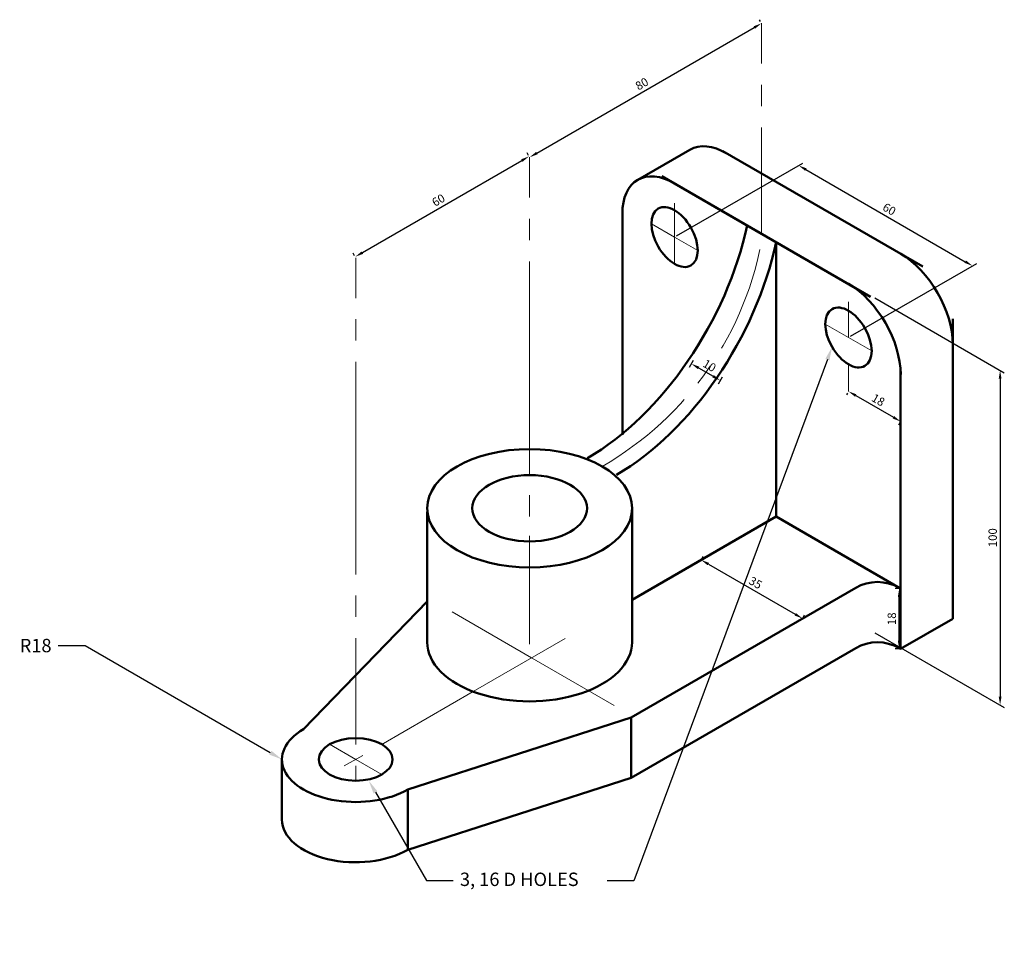
# Model space of a CAD drawing. Units: millimetres. Extents: x 10284 to 10578, y 6421 to 6701.
import ezdxf
from ezdxf import colors
from ezdxf.entities.mleader import LeaderData, LeaderLine
from ezdxf.math import Vec2, Vec3

# ---------------------------------------------------------------- set-up
doc = ezdxf.new("R2010")
doc.units = ezdxf.units.MM
doc.linetypes.add('CENTER', pattern=[50.8, 31.75, -6.35, 6.35, -6.35])
for name, color, linetype, lineweight in [('M-CNTR', 4, 'CENTER', 18), ('M-DIMS', 2, 'Continuous', 25), ('M-OUTL', 7, 'Continuous', 50), ('M-TEXT', 3, 'Continuous', 25)]:
    doc.layers.add(name, color=color, linetype=linetype, lineweight=lineweight)
doc.styles.get("Standard").update_dxf_attribs({"font": 'arial.ttf'})
doc.dimstyles.new('ISO-25', dxfattribs={"dimtxt": 2.5, "dimasz": 2.5, "dimexe": 1.25, "dimexo": 0.625, "dimtad": 1, "dimtxsty": 'Standard', "dimcen": 2.5, "dimadec": 0, "dimazin": 0, "dimtfac": 1, "dimtmove": 0, "dimatfit": 3, "dimfxl": 1, "dimarcsym": 0})

# ---------------------------------------------------------------- blocks, each defined once
blk = doc.blocks.new('*D1')
at = {"layer": 'Defpoints', "color": 0, "transparency": 16777216}
for p in [(10546.86, 6530.7), (10547.29, 6530.7), (10547.29, 6512.7)]:
    blk.add_point(p, dxfattribs=at)
at = {"layer": 'M-DIMS', "color": 0, "lineweight": -2, "transparency": 16777216}
for p, q in [((10546.66, 6530.7), (10545.61, 6530.7)), ((10546.86, 6515.2), (10546.86, 6528.2)), ((10546.66, 6512.7), (10545.61, 6512.7))]:
    blk.add_line(p, q, dxfattribs=at)
at = {"layer": 'M-DIMS', "color": 0, "transparency": 16777216}
for points in [[(10546.44, 6528.2), (10547.28, 6528.2), (10546.86, 6530.7)], [(10546.44, 6515.2), (10547.28, 6515.2), (10546.86, 6512.7)]]:
    blk.add_solid(points, dxfattribs=at)
at = {"layer": 'M-DIMS', "color": 0, "transparency": 16777216, "insert": (10544.96, 6521.7), "char_height": 2.5, "attachment_point": 5, "rotation": 90}
blk.add_mtext('18', dxfattribs=at)
blk = doc.blocks.new('*D2')
at = {"layer": 'Defpoints', "color": 0, "transparency": 16777216}
for p in [(10487.67, 6539.28), (10517.98, 6521.78), (10517.98, 6521.78)]:
    blk.add_point(p, dxfattribs=at)
at = {"layer": 'M-DIMS', "color": 0, "lineweight": -2, "transparency": 16777216}
for p, q in [((10487.98, 6539.82), (10488.29, 6540.36)), ((10489.83, 6538.03), (10515.81, 6523.03)), ((10518.29, 6522.32), (10518.6, 6522.86))]:
    blk.add_line(p, q, dxfattribs=at)
at = {"layer": 'M-DIMS', "color": 0, "transparency": 16777216}
for points in [[(10490.04, 6538.39), (10489.63, 6537.67), (10487.67, 6539.28)], [(10516.02, 6523.39), (10515.61, 6522.67), (10517.98, 6521.78)]]:
    blk.add_solid(points, dxfattribs=at)
at = {"layer": 'M-DIMS', "color": 0, "transparency": 16777216, "insert": (10503.77, 6532.18), "char_height": 2.5, "attachment_point": 5, "rotation": 330}
blk.add_mtext('35', dxfattribs=at)
blk = doc.blocks.new('*D3')
at = {"layer": 'Defpoints', "color": 0, "transparency": 16777216}
for p in [(10531.7, 6589.62), (10547.29, 6580.62), (10547.29, 6580.62)]:
    blk.add_point(p, dxfattribs=at)
at = {"layer": 'M-DIMS', "color": 0, "lineweight": -2, "transparency": 16777216}
for p, q in [((10531.39, 6589.08), (10531.07, 6588.54)), ((10533.86, 6588.37), (10545.12, 6581.87)), ((10546.98, 6580.08), (10546.66, 6579.54))]:
    blk.add_line(p, q, dxfattribs=at)
at = {"layer": 'M-DIMS', "color": 0, "transparency": 16777216}
for points in [[(10534.07, 6588.73), (10533.66, 6588.01), (10531.7, 6589.62)], [(10545.33, 6582.23), (10544.91, 6581.51), (10547.29, 6580.62)]]:
    blk.add_solid(points, dxfattribs=at)
at = {"layer": 'M-DIMS', "color": 0, "transparency": 16777216, "insert": (10540.44, 6586.77), "char_height": 2.5, "attachment_point": 5, "rotation": 330}
blk.add_mtext('18', dxfattribs=at)
blk = doc.blocks.new('*D4')
at = {"layer": 'Defpoints', "color": 0, "transparency": 16777216}
for p in [(10479.74, 6635.7), (10568.76, 6627.1), (10531.7, 6605.7)]:
    blk.add_point(p, dxfattribs=at)
at = {"layer": 'M-DIMS', "color": 0, "lineweight": -2, "transparency": 16777216}
for p, q in [((10480.36, 6636.06), (10518.05, 6657.82)), ((10518.97, 6655.85), (10566.6, 6628.35)), ((10532.32, 6606.06), (10570.01, 6627.82))]:
    blk.add_line(p, q, dxfattribs=at)
at = {"layer": 'M-DIMS', "color": 0, "transparency": 16777216}
for points in [[(10519.18, 6656.21), (10518.76, 6655.49), (10516.8, 6657.1)], [(10566.81, 6628.71), (10566.39, 6627.99), (10568.76, 6627.1)]]:
    blk.add_solid(points, dxfattribs=at)
at = {"layer": 'M-DIMS', "color": 0, "transparency": 16777216, "insert": (10543.73, 6643.75), "char_height": 2.5, "attachment_point": 5, "rotation": 330}
blk.add_mtext('60', dxfattribs=at)
blk = doc.blocks.new('*D5')
at = {"layer": 'Defpoints', "color": 0, "transparency": 16777216}
for p in [(10485.59, 6599.35), (10493.4, 6592.87), (10494.25, 6594.35)]:
    blk.add_point(p, dxfattribs=at)
at = {"layer": 'M-DIMS', "color": 0, "lineweight": -2, "transparency": 16777216}
for p, q in [((10485.28, 6598.81), (10484.12, 6596.79)), ((10486.91, 6596.62), (10491.24, 6594.12)), ((10493.94, 6593.81), (10492.78, 6591.79))]:
    blk.add_line(p, q, dxfattribs=at)
at = {"layer": 'M-DIMS', "color": 0, "transparency": 16777216}
for points in [[(10487.12, 6596.99), (10486.7, 6596.26), (10484.74, 6597.87)], [(10491.45, 6594.49), (10491.03, 6593.76), (10493.4, 6592.87)]]:
    blk.add_solid(points, dxfattribs=at)
at = {"layer": 'M-DIMS', "color": 0, "transparency": 16777216, "insert": (10490.02, 6597.02), "char_height": 2.5, "attachment_point": 5, "rotation": 330}
blk.add_mtext('10', dxfattribs=at)
blk = doc.blocks.new('*D6')
at = {"layer": 'Defpoints', "color": 0, "transparency": 16777216}
for p in [(10538.91, 6617.9), (10538.91, 6517.9), (10577, 6495.91)]:
    blk.add_point(p, dxfattribs=at)
at = {"layer": 'M-DIMS', "color": 0, "lineweight": -2, "transparency": 16777216}
for p, q in [((10539.54, 6617.54), (10578.25, 6595.18)), ((10577, 6593.41), (10577, 6498.41)), ((10539.54, 6517.54), (10578.25, 6495.18))]:
    blk.add_line(p, q, dxfattribs=at)
at = {"layer": 'M-DIMS', "color": 0, "transparency": 16777216}
for points in [[(10576.59, 6593.41), (10577.42, 6593.41), (10577, 6595.91)], [(10576.59, 6498.41), (10577.42, 6498.41), (10577, 6495.91)]]:
    blk.add_solid(points, dxfattribs=at)
at = {"layer": 'M-DIMS', "color": 0, "transparency": 16777216, "insert": (10575.1, 6545.91), "char_height": 2.5, "attachment_point": 5, "rotation": 90}
blk.add_mtext('100', dxfattribs=at)
blk = doc.blocks.new('*D7')
at = {"layer": 'Defpoints', "color": 0, "transparency": 16777216}
for p in [(10505.72, 6699.54), (10505.72, 6699.54), (10436.44, 6659.54)]:
    blk.add_point(p, dxfattribs=at)
at = {"layer": 'M-DIMS', "color": 0, "lineweight": -2, "transparency": 16777216}
for p, q in [((10438.6, 6660.79), (10503.55, 6698.29)), ((10505.41, 6700.08), (10505.09, 6700.62)), ((10436.12, 6660.08), (10435.81, 6660.62))]:
    blk.add_line(p, q, dxfattribs=at)
at = {"layer": 'M-DIMS', "color": 0, "transparency": 16777216}
for points in [[(10503.35, 6698.65), (10503.76, 6697.93), (10505.72, 6699.54)], [(10438.39, 6661.15), (10438.81, 6660.43), (10436.44, 6659.54)]]:
    blk.add_solid(points, dxfattribs=at)
at = {"layer": 'M-DIMS', "color": 0, "transparency": 16777216, "insert": (10470.13, 6681.19), "char_height": 2.5, "attachment_point": 5, "rotation": 30}
blk.add_mtext('80', dxfattribs=at)
blk = doc.blocks.new('*D8')
at = {"layer": 'Defpoints', "color": 0, "transparency": 16777216}
for p in [(10436.28, 6659.81), (10436.44, 6659.54), (10384.48, 6629.54)]:
    blk.add_point(p, dxfattribs=at)
at = {"layer": 'M-DIMS', "color": 0, "lineweight": -2, "transparency": 16777216}
for p, q in [((10436.12, 6660.08), (10435.66, 6660.89)), ((10386.49, 6631.06), (10434.12, 6658.56)), ((10384.16, 6630.08), (10383.7, 6630.89))]:
    blk.add_line(p, q, dxfattribs=at)
at = {"layer": 'M-DIMS', "color": 0, "transparency": 16777216}
for points in [[(10433.91, 6658.92), (10434.33, 6658.2), (10436.28, 6659.81)], [(10386.28, 6631.42), (10386.69, 6630.7), (10384.32, 6629.81)]]:
    blk.add_solid(points, dxfattribs=at)
at = {"layer": 'M-DIMS', "color": 0, "transparency": 16777216, "insert": (10409.35, 6646.45), "char_height": 2.5, "attachment_point": 5, "rotation": 30}
blk.add_mtext('60', dxfattribs=at)

msp = doc.modelspace()

# ---------------------------------------------------------------- linework, layer by layer
at = {"layer": 'M-CNTR'}
for p, q in [((10505.719, 6636.703), (10505.719, 6699.54)), ((10436.437, 6596.703), (10436.437, 6659.54)), ((10479.738, 6635.703), (10479.738, 6645.85)), ((10479.738, 6635.703), (10472.81, 6639.703)), ((10479.738, 6635.703), (10479.738, 6627.703)), ((10486.666, 6631.703), (10479.738, 6635.703)), ((10384.475, 6566.703), (10384.475, 6629.54)), ((10531.699, 6605.703), (10531.699, 6616.342)), ((10531.699, 6605.703), (10524.771, 6609.703)), ((10531.699, 6605.703), (10538.628, 6601.703)), ((10436.437, 6596.703), (10436.437, 6509.703)), ((10531.699, 6597.703), (10531.699, 6589.619)), ((10384.475, 6566.703), (10384.475, 6473.339)), ((10436.437, 6514.703), (10436.437, 6554.703)), ((10510.049, 6552.203), (10467.055, 6527.381)), ((10437.03, 6510.046), (10413.303, 6523.745)), ((10419.554, 6499.955), (10452.133, 6518.765)), ((10435.843, 6510.731), (10461.727, 6495.787)), ((10419.554, 6499.955), (10377.892, 6475.902)), ((10384.475, 6479.703), (10376.681, 6484.203)), ((10384.475, 6479.703), (10392.269, 6475.203))]:
    msp.add_line(p, q, dxfattribs=at)
msp.add_arc((10409.237, 6652.306), 98.127, 299.85624, 350.72636, dxfattribs=at)
at = {"layer": 'M-OUTL'}
for p, q in [((10468.719, 6652.795), (10484.307, 6661.795)), ((10553.876, 6626.899), (10494.111, 6661.404)), ((10505.719, 6636.703), (10475.978, 6653.874)), ((10475.978, 6653.874), (10538.288, 6617.899)), ((10464.149, 6576.661), (10464.149, 6644.652)), ((10510.049, 6634.203), (10501.389, 6639.203)), ((10505.719, 6636.703), (10510.049, 6634.203)), ((10510.049, 6634.203), (10510.049, 6552.203)), ((10562.876, 6521.703), (10562.876, 6611.311)), ((10547.288, 6596.703), (10547.288, 6512.703)), ((10467.055, 6514.7), (10467.055, 6554.703)), ((10467.055, 6554.703), (10467.055, 6514.703)), ((10405.868, 6553.689), (10405.818, 6514.716)), ((10467.059, 6527.381), (10510.052, 6552.203)), ((10510.049, 6552.203), (10547.074, 6530.826)), ((10466.748, 6492.203), (10533.86, 6530.95)), ((10546.86, 6530.95), (10547.288, 6530.703)), ((10547.288, 6512.703), (10547.288, 6530.703)), ((10368.887, 6488.703), (10405.834, 6526.901)), ((10547.288, 6512.703), (10562.876, 6521.703)), ((10466.748, 6474.203), (10533.86, 6512.95)), ((10546.86, 6512.95), (10547.288, 6512.703)), ((10466.748, 6492.203), (10400.064, 6470.703)), ((10466.751, 6474.203), (10466.751, 6492.203)), ((10362.43, 6461.703), (10362.43, 6479.703)), ((10400.064, 6452.703), (10466.748, 6474.203)), ((10400.067, 6452.703), (10400.067, 6470.703))]:
    msp.add_line(p, q, dxfattribs=at)
for centre in [(10540.36, 6519.692), (10540.36, 6501.692)]:
    msp.add_arc(centre, 13, 60, 120, dxfattribs=at)
for centre, major_axis, start_param, end_param in [((10495.33, 6642.703), (-11.023, 19.092), 5.4977871, 6.2831853), ((10479.741, 6633.703), (-11.023, 19.092), 5.4977871, 6.2831853), ((10479.741, 6633.703), (-11.023, 19.092), 0, 0.7853982), ((10453.767, 6626.709), (34.906, 60.46), 3.9268553, 5.2314692), ((10462.428, 6621.709), (34.906, 60.46), 3.9268553, 5.2314692), ((10547.291, 6612.703), (11.023, -19.092), 0.7853982, 2.3561945), ((10531.703, 6603.703), (11.023, -19.092), 0.7853982, 2.3561945), ((10436.437, 6514.703), (-30.619, 0), 6.2824387, 9.4249273), ((10384.475, 6479.703), (-22.045, 0), 5.4977871, 8.6393798), ((10384.475, 6461.703), (-22.045, 0), 6.2831853, 8.6393798)]:
    msp.add_ellipse(centre, major_axis=major_axis, ratio=0.5773503, start_param=start_param, end_param=end_param, dxfattribs=at)
for centre, major_axis in [((10479.738, 6635.703), (4.899, -8.485)), ((10531.699, 6605.703), (4.899, -8.485)), ((10436.437, 6554.703), (-30.619, 0)), ((10436.437, 6554.703), (-17.146, 0)), ((10384.475, 6479.703), (-11.023, 0))]:
    msp.add_ellipse(centre, major_axis=major_axis, ratio=0.5773503, dxfattribs=at)

# ---------------------------------------------------------------- dimensions: what is measured, and where the dimension line sits
at = {"layer": 'M-DIMS'}
for base, p1, p2, picture, middle in [((10505.719, 6699.54), (10436.437, 6659.54), (10505.719, 6699.54), '*D7', (10470.127, 6681.186)), ((10436.283, 6659.806), (10384.475, 6629.54), (10436.437, 6659.54), '*D8', (10409.351, 6646.453))]:
    dim = msp.add_linear_dim(base=base, p1=p1, p2=p2, angle=30, dimstyle='ISO-25', override={"dimrnd": 0}, dxfattribs=at)
    dim.commit()
    dim.dimension.update_dxf_attribs({"geometry": picture, "text_midpoint": middle})
for p1, p2, distance, picture, middle in [((10479.738, 6635.703), (10531.699, 6605.703), 37.066, '*D4', (10543.735, 6643.749)), ((10538.913, 6617.899), (10538.913, 6517.899), 38.092, '*D6', (10575.103, 6545.907)), ((10485.594, 6599.348), (10494.255, 6594.348), -1.701, '*D5', (10490.025, 6597.021)), ((10531.699, 6589.619), (10547.288, 6580.619), 0, '*D3', (10540.444, 6586.766)), ((10487.668, 6539.281), (10517.979, 6521.781), 0, '*D2', (10503.775, 6532.179)), ((10547.288, 6512.703), (10547.288, 6530.703), 0.428, '*D1', (10544.958, 6521.703))]:
    dim = msp.add_aligned_dim(p1=p1, p2=p2, distance=distance, dimstyle='ISO-25', override={"dimclrd": 0, "dimclre": 0, "dimclrt": 0}, dxfattribs=at)
    dim.commit()
    dim.dimension.update_dxf_attribs({"geometry": picture, "text_midpoint": middle})

# ---------------------------------------------------------------- leaders
at = {"layer": 'M-TEXT'}
ml = msp.add_multileader_mtext('Standard', dxfattribs=at)
ml.set_content('', color=256)
ml.set_leader_properties()
ml.build(insert=Vec2(0, 0))
ctx = ml.context
ctx.base_point, ctx.plane_origin = Vec3(10455.571, 6443.479), Vec3(10526.8, 6602.874)
ctx.text_align_type = 2
notes = []
notes.append((ctx, [(0, (1, 1, 0), (10467.571, 6443.479), (-1, 0), 8, [(0, [(10526.8, 6602.874)], 0, [])])]))
ctx.mtext.insert, ctx.mtext.alignment, ctx.mtext.flow_direction = Vec3(10457.571, 6445.479), 3, 5
ml = msp.add_multileader_mtext('Standard', dxfattribs=at)
ml.set_content('R18', color=256)
ml.set_leader_properties()
ml.build(insert=Vec2(0, 0))
ctx = ml.context
ctx.base_point, ctx.plane_origin = Vec3(10282.042, 6513.664), Vec3(10362.43, 6479.703)
ctx.text_align_type = 2
notes.append((ctx, [(0, (1, 1, 0), (10303.608, 6513.664), (-1, 0), 8, [(0, [(10362.43, 6479.703)], 0, [])])]))
ctx.mtext.insert, ctx.mtext.alignment, ctx.mtext.flow_direction = Vec3(10293.608, 6515.698), 3, 5
ml = msp.add_multileader_mtext('Standard', dxfattribs=at)
ml.set_content('3, 16 D HOLES', color=256)
ml.set_leader_properties()
ml.build(insert=Vec2(0, 0))
ctx = ml.context
ctx.base_point, ctx.plane_origin = Vec3(10413.607, 6443.488), Vec3(10388.372, 6473.339)
notes.append((ctx, [(0, (1, 1, 0), (10405.607, 6443.488), (1, 0), 8, [(0, [(10388.372, 6473.339)], 0, [])])]))
ctx.mtext.insert, ctx.mtext.flow_direction = Vec3(10415.607, 6445.884), 5
for ctx, leaders in notes:
    for number, flags, end, landing, length, lines in leaders:
        leader = LeaderData()
        leader.index, (leader.has_last_leader_line, leader.has_dogleg_vector, leader.attachment_direction) = number, flags
        leader.last_leader_point, leader.dogleg_vector, leader.dogleg_length = Vec3(end), Vec3(landing), length
        for number, points, colour, breaks in lines:
            line = LeaderLine()
            line.index, line.vertices, line.color, line.breaks = number, Vec3.list(points), colors.encode_raw_color(colour), breaks
            leader.lines.append(line)
        ctx.leaders.append(leader)

doc.saveas('drawing.dxf')
